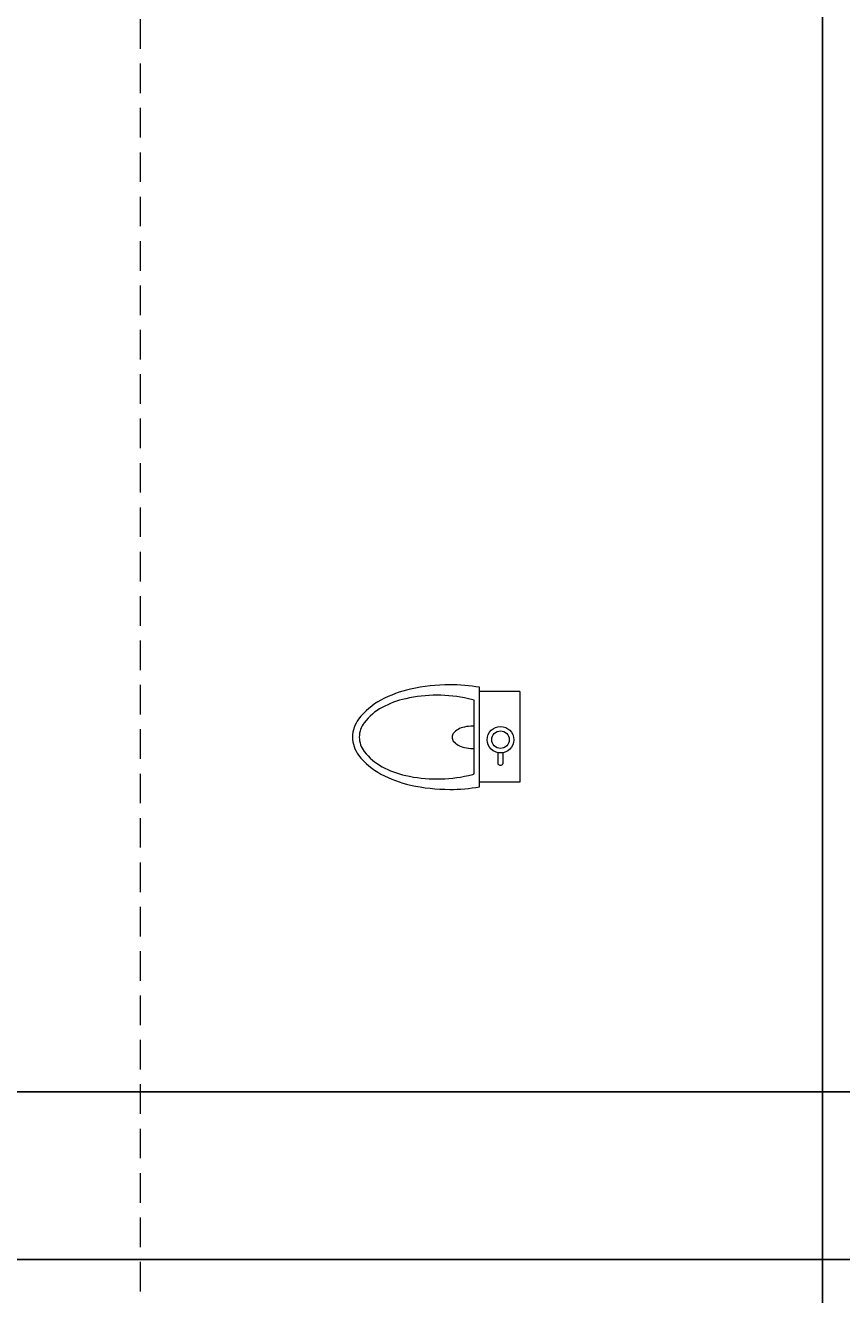
# Model space of a CAD drawing. Units: inches. Extents: x 1770 to 2988, y 1161 to 3221.
# Tile 30 of 44: x 2631 to 2807, y 2095 to 2368. Entities that reach past the tile are written whole.
import ezdxf

# ---------------------------------------------------------------- set-up
doc = ezdxf.new("R2010")
doc.units = ezdxf.units.IN
doc.linetypes.add('DASHED2', pattern=[9.525, 6.35, -3.175])
for name, color, linetype, lineweight in [('A-ANNO-DIMS', 2, 'Continuous', 18), ('A-FLOR-FIXT', 9, 'Continuous', 18), ('A-ROOF-OVHD', 7, 'DASHED2', 18), ('C-PROP', 7, 'Continuous', 25)]:
    doc.layers.add(name, color=color, linetype=linetype, lineweight=lineweight)
doc.styles.get("Standard").update_dxf_attribs({"font": 'arial.ttf'})
doc.dimstyles.get("Standard").update_dxf_attribs({"dimtxt": 0.18, "dimasz": 0.18, "dimexe": 0.18, "dimexo": 0.0625, "dimgap": 0.09, "dimtad": 0, "dimtih": 1, "dimtoh": 1, "dimdec": 4, "dimzin": 0, "dimdsep": 46, "dimtxsty": 'Standard', "dimcen": 0.09, "dimadec": 0, "dimazin": 0, "dimtfac": 1, "dimtdec": 4, "dimtofl": 0, "dimtmove": 0, "dimatfit": 3, "dimfxl": 1, "dimtolj": 1, "dimtzin": 0, "dimarcsym": 0})

# ---------------------------------------------------------------- blocks, each defined once
blk = doc.blocks.new('A$C7FD35E1A')
for p, q in [((0.0233, 0.5799), (0.0233, 0.4408)), ((0.0233, 0.5799), (0.338, 0.5799)), ((0.338, 0.5799), (0.338, 0.4408)), ((0.2356, 0.5044), (0.275, 0.5044)), ((0.2357, 0.5217), (0.2745, 0.5217)), ((0.3542, 0.4408), (0.0087, 0.4408)), ((0.3093, 0.4224), (0.0536, 0.4224))]:
    blk.add_line(p, q)
for radius in [0.046, 0.0305]:
    blk.add_circle((0.1904, 0.5132), radius)
for centre, radius, start, end in [((0.2685, 0.5129), 0.0107, 307.488, 55.394), ((0.6238, 0.337), 0.6238, 170.4184, 180), ((-0.261, 0.337), 0.6238, 0, 9.5816), ((0.5354, 0.2931), 0.4991, 167.4267, 180), ((0.3603, 0.3321), 0.3197, 163.5954, 167.4267), ((0.277, 0.4171), 0.1337, 177.7133, 180), ((0.277, 0.4171), 0.1337, 180, 192.5399), ((0.0869, 0.4171), 0.1337, 347.4601, 0), ((0.0869, 0.4171), 0.1337, 360, 2.2867), ((0.0026, 0.3321), 0.3197, 12.5733, 16.4046), ((-0.1725, 0.2931), 0.4991, 0, 12.5733), ((0.23, 0.4066), 0.0855, 192.5399, 208.2349), ((0.2004, 0.3907), 0.052, 208.2349, 232.3543), ((0.1635, 0.3907), 0.052, 307.6457, 331.7651), ((0.1339, 0.4066), 0.0855, 331.7651, 347.4601), ((0.6238, 0.337), 0.6238, 180, 192.5733), ((0.182, 0.3668), 0.0218, 232.3543, 270), ((0.182, 0.3668), 0.0218, 270, 307.6457), ((-0.261, 0.337), 0.6238, 347.4267, 0), ((0.5354, 0.2931), 0.4991, 180, 192.5733), ((-0.1725, 0.2931), 0.4991, 347.4267, 0), ((0.405, 0.2881), 0.3996, 192.5733, 208.3008), ((0.3603, 0.254), 0.3197, 192.5733, 208.3008), ((0.0026, 0.254), 0.3197, 331.6992, 347.4267), ((-0.0421, 0.2881), 0.3996, 331.6992, 347.4267), ((0.2672, 0.214), 0.2432, 208.3008, 232.4306), ((0.2501, 0.1947), 0.1945, 208.3008, 232.4306), ((0.1128, 0.1947), 0.1945, 307.5694, 331.6992), ((0.0957, 0.214), 0.2432, 307.5694, 331.6992), ((0.1814, 0.1024), 0.1024, 232.4306, 270), ((0.1814, 0.1055), 0.082, 232.4306, 270), ((0.1814, 0.1055), 0.082, 270, 307.5694), ((0.1814, 0.1024), 0.1024, 270, 307.5694)]:
    blk.add_arc(centre, radius, start, end)
blk = doc.blocks.new('*D61')
at = {"layer": 'A-ANNO-DIMS', "color": 0, "lineweight": -2, "transparency": 16777216}
for p, q in [((2625.76, 2376.7), (2866.87, 2376.7)), ((2866.69, 2376.52), (2866.69, 1993.63)), ((2866.69, 1610.38), (2866.69, 1993.27)), ((2625.76, 1610.2), (2866.87, 1610.2))]:
    blk.add_line(p, q, dxfattribs=at)
at = {"layer": 'A-ANNO-DIMS', "color": 0, "transparency": 16777216}
for points in [[(2866.66, 2376.52), (2866.72, 2376.52), (2866.69, 2376.7)], [(2866.66, 1610.38), (2866.72, 1610.38), (2866.69, 1610.2)]]:
    blk.add_solid(points, dxfattribs=at)
at = {"layer": 'Defpoints', "color": 0, "transparency": 16777216}
for p in [(2625.7, 2376.7), (2866.69, 2376.7), (2625.7, 1610.2)]:
    blk.add_point(p, dxfattribs=at)
at = {"layer": 'A-ANNO-DIMS', "color": 0, "transparency": 16777216, "insert": (2866.69, 1993.45), "char_height": 0.18, "attachment_point": 5}
blk.add_mtext('\\A1;766.5', dxfattribs=at)
blk = doc.blocks.new('*D89')
at = {"layer": 'A-ANNO-DIMS', "color": 0, "lineweight": -2, "transparency": 16777216}
for p, q in [((2160.76, 2138.84), (2866.87, 2138.84)), ((2866.69, 2138.66), (2866.69, 2121.02)), ((2866.69, 2103.02), (2866.69, 2120.66)), ((2160.76, 2102.84), (2866.87, 2102.84))]:
    blk.add_line(p, q, dxfattribs=at)
at = {"layer": 'A-ANNO-DIMS', "color": 0, "transparency": 16777216}
for points in [[(2866.66, 2138.66), (2866.72, 2138.66), (2866.69, 2138.84)], [(2866.66, 2103.02), (2866.72, 2103.02), (2866.69, 2102.84)]]:
    blk.add_solid(points, dxfattribs=at)
at = {"layer": 'Defpoints', "color": 0, "transparency": 16777216}
for p in [(2160.7, 2138.84), (2866.69, 2138.84), (2160.7, 2102.84)]:
    blk.add_point(p, dxfattribs=at)
at = {"layer": 'A-ANNO-DIMS', "color": 0, "transparency": 16777216, "insert": (2866.69, 2120.84), "char_height": 0.18, "attachment_point": 5}
blk.add_mtext('\\A1;36', dxfattribs=at)

msp = doc.modelspace()

# ---------------------------------------------------------------- linework, layer by layer
at = {"layer": 'A-ROOF-OVHD'}
msp.add_line((2656.0216, 1610.2021), (2656.0216, 2405.7876), dxfattribs=at)
at = {"layer": 'C-PROP'}
msp.add_lwpolyline([(1971.5344, 2506.2747), (2802.4374, 2506.2747), (2802.4374, 1323.5288), (1971.5344, 1323.5288)], close=True, dxfattribs=at)

# ---------------------------------------------------------------- block references
at = {"layer": 'A-FLOR-FIXT', "xscale": 61.88350044382122, "yscale": 61.88350044382122, "zscale": 61.88350044382122, "rotation": 270}
msp.add_blockref('A$C7FD35E1A', (2701.5485, 2226.1783), dxfattribs=at)

# ---------------------------------------------------------------- dimensions: what is measured, and where the dimension line sits
at = {"layer": 'A-ANNO-DIMS'}
for base, p1, p2, override, picture, middle in [((2866.6874, 2376.7021), (2625.696, 1610.2021), (2625.696, 2376.7021), {"dimdec": 1, "dimlfac": 1, "dimrnd": 0, "dimzin": 0, "dimdsep": 46, "dimlunit": 2}, '*D61', (2866.6874, 1993.4521)), ((2866.6874, 2138.8392), (2160.696, 2102.8392), (2160.696, 2138.8392), {"dimdec": 0, "dimlfac": 1, "dimrnd": 0, "dimzin": 0, "dimdsep": 46, "dimlunit": 2}, '*D89', (2866.6874, 2120.8392))]:
    dim = msp.add_linear_dim(base=base, p1=p1, p2=p2, angle=90, dimstyle='Standard', override=override, dxfattribs=at)
    dim.commit()
    dim.dimension.update_dxf_attribs({"geometry": picture, "text_midpoint": middle})

doc.saveas('drawing.dxf')
